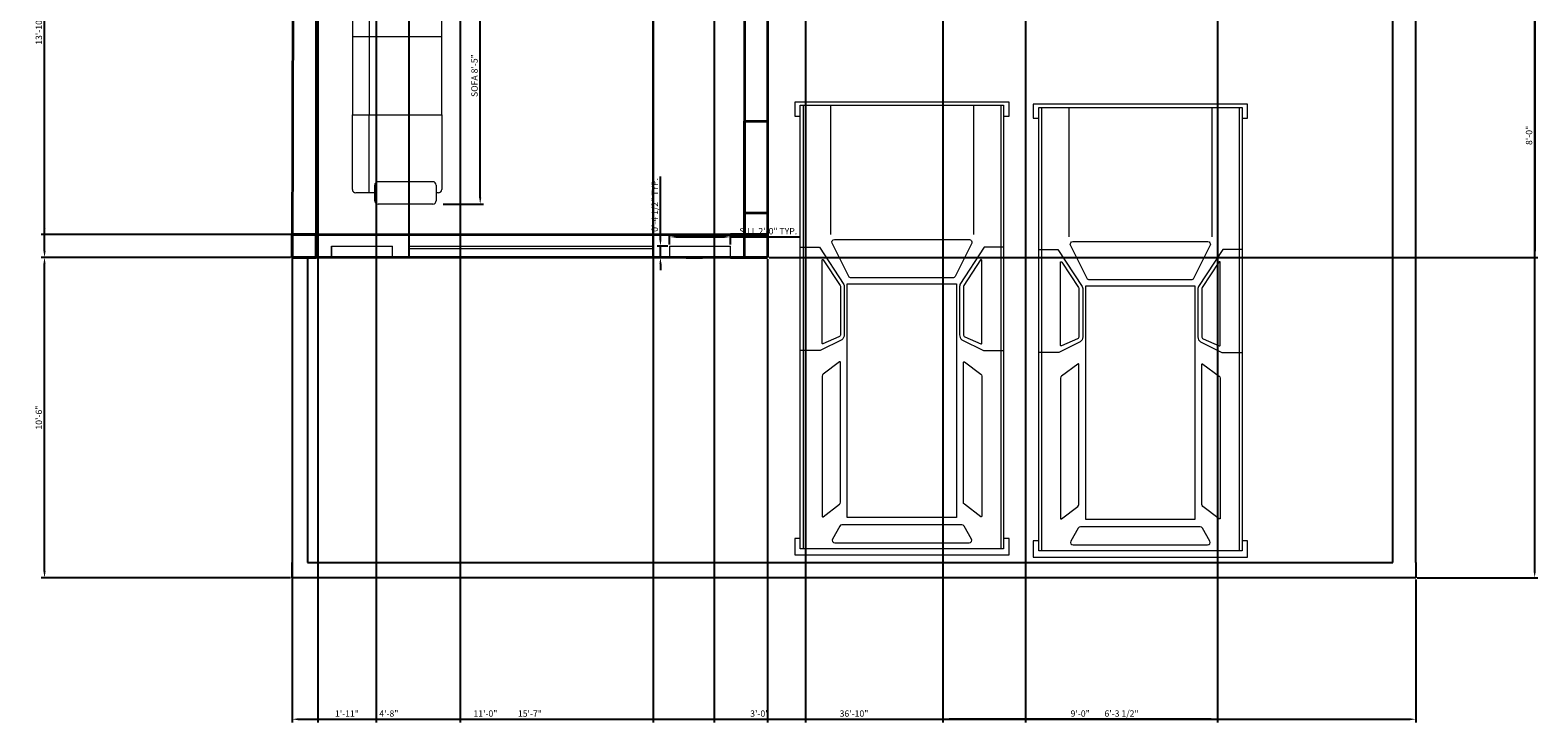
# Model space of a CAD drawing. Units: inches. Extents: x 1624 to 3956, y 1589 to 5028.
# Tile 1 of 16: x 1624 to 2218, y 1589 to 1862. Entities that reach past the tile are written whole.
import ezdxf

# ---------------------------------------------------------------- set-up
doc = ezdxf.new("R2010")
doc.units = ezdxf.units.IN
for name, color, linetype, lineweight in [('A-ANNO-DIMS', 2, 'Continuous', 13), ('A-COLS', 1, 'Continuous', 40), ('A-EQPM-VEHI', 8, 'Continuous', 13), ('A-FURN', 8, 'Continuous', 18), ('A-GLAZ', 4, 'Continuous', 18), ('A-WALL', 7, 'Continuous', 35), ('C-PROP', 7, 'Continuous', 25)]:
    doc.layers.add(name, color=color, linetype=linetype, lineweight=lineweight)
doc.styles.get("Standard").update_dxf_attribs({"font": 'arial.ttf'})
doc.dimstyles.new('Copy of ISO-25', dxfattribs={"dimtxt": 2.5, "dimasz": 2.5, "dimexe": 1.25, "dimexo": 0.625, "dimtad": 1, "dimdec": 1, "dimlunit": 4, "dimtxsty": 'Standard', "dimcen": 2.5, "dimadec": 0, "dimazin": 0, "dimtfac": 1, "dimtdec": 1, "dimtmove": 0, "dimatfit": 3, "dimfxl": 1, "dimarcsym": 0})

# ---------------------------------------------------------------- blocks, each defined once
blk = doc.blocks.new('*U16')
for p, q in [((32, 987), (4462, 987)), ((32, 715), (1324, 715)), ((32, -715), (1324, -715)), ((32, -987), (4462, -987))]:
    blk.add_line(p, q)
for points in [[(141, 1016), (141, 1071), (0, 1071), (0, -1071), (141, -1071), (141, -1016), (32, -1016), (32, 1016)], [(4362, 1016), (4462, 1016), (4462, -1016), (4362, -1016), (4362, -1071), (4525, -1071), (4525, 1071), (4362, 1071)], [(32, 1016), (4462, 1016), (4462, -1016), (32, -1016)], [(1815, 546), (4151, 546), (4151, -546), (1815, -546)]]:
    blk.add_lwpolyline(points, close=True)
for points in [[(1451, 1016), (1451, 823), (1822, 580, 0.086577), (1843, 576), (2326, 576, 0.227875), (2376, 600), (2482, 816), (2482, 1016)], [(1451, -1016), (1451, -823), (1822, -580, -0.086577), (1843, -576), (2326, -576, -0.227875), (2376, -600), (2482, -816), (2482, -1016)]]:
    blk.add_lwpolyline(points, format="xyb")
for points in [[(1577, 786), (1832, 618, 0.146139), (1846, 614), (2322, 614, 0.29766), (2345, 629), (2415, 789, 0.541236), (2409, 798), (1580, 798, 0.744989)], [(2596, 624), (2717, 787, -0.236929), (2737, 798), (4138, 798, -0.621576), (4143, 787), (4018, 624, -0.233368), (3998, 614), (2601, 614, -0.616908)], [(1410, 697), (1742, 531, -0.284287), (1756, 508), (1756, -508, -0.284287), (1742, -531), (1410, -697, -0.557284), (1373, -674), (1373, 674, -0.557284)], [(4366, 694), (4237, 622, 0.271143), (4224, 599), (4224, -599, 0.271143), (4237, -622), (4366, -694, 0.573387), (4404, -672), (4404, 672, 0.573387)], [(1577, -786), (1832, -618, -0.146139), (1846, -614), (2322, -614, -0.29766), (2345, -629), (2415, -789, -0.541236), (2409, -798), (1580, -798, -0.744989)], [(2596, -624), (2717, -787, 0.236929), (2737, -798), (4138, -798, 0.621576), (4143, -787), (4018, -624, 0.233368), (3998, -614), (2601, -614, 0.616908)]]:
    blk.add_lwpolyline(points, format="xyb", close=True)
blk = doc.blocks.new('A$C555E41E5')
for p, q in [((0.1, 0.6), (0.1, 0.77)), ((0.13, 0.8), (0.8, 0.8)), ((0.8, 0.8), (0.8, 0)), ((0.8, 0.8), (0.8, 0)), ((1.5, 0.8), (0.8, 0.8)), ((2.17, 0.8), (1.5, 0.8)), ((1.5, 0.8), (1.5, 0)), ((1.5, 0.8), (1.5, 0)), ((2.2, 0.6), (2.2, 0.77)), ((0, 0.08), (0, 0.57)), ((0.03, 0.6), (0.17, 0.6)), ((0.1, 0.65), (0.8, 0.65)), ((0.2, 0.08), (0.2, 0.57)), ((1.53, 0.65), (0.8, 0.65)), ((2.2, 0.65), (1.5, 0.65)), ((2.1, 0.08), (2.1, 0.57)), ((2.27, 0.6), (2.13, 0.6)), ((2.3, 0.08), (2.3, 0.57)), ((0.17, 0.05), (0.03, 0.05)), ((0.1, 0.03), (0.1, 0.05)), ((0.8, 0), (0.13, 0)), ((0.8, 0), (1.5, 0)), ((1.5, 0), (2.17, 0)), ((2.13, 0.05), (2.27, 0.05)), ((2.2, 0.03), (2.2, 0.05))]:
    blk.add_line(p, q)
for centre, start, end in [((0.13, 0.77), 90, 180), ((2.17, 0.77), 0, 90), ((0.03, 0.57), 90, 180), ((0.17, 0.57), 0, 90), ((2.13, 0.57), 90, 180), ((2.27, 0.57), 0, 90), ((0.03, 0.08), 180, 270), ((0.13, 0.03), 180, 270), ((0.17, 0.08), 270, 0), ((2.13, 0.08), 180, 270), ((2.17, 0.03), 270, 0), ((2.27, 0.08), 270, 0)]:
    blk.add_arc(centre, 0.03, start, end)
blk = doc.blocks.new('A$C2BCD7A6E')
blk.add_blockref('A$C555E41E5', (0, 0))
blk = doc.blocks.new('SILL-RECESS-24IN')
for p, q in [((0, 4.5), (0, 0)), ((0, 4.5), (24, 4.5)), ((24, 0), (24, 4.5))]:
    blk.add_line(p, q)
blk = doc.blocks.new('*D58')
at = {"layer": 'A-ANNO-DIMS', "color": 0, "lineweight": -2, "transparency": 16777216}
for p, q in [((1876.03, 1777.92), (1876.03, 1782.14)), ((1878.53, 1780.89), (1897.53, 1780.89)), ((1900.03, 1777.92), (1900.03, 1782.14)), ((1900.03, 1780.89), (1927.16, 1780.89))]:
    blk.add_line(p, q, dxfattribs=at)
at = {"layer": 'A-ANNO-DIMS', "color": 0, "transparency": 16777216}
for points in [[(1878.53, 1781.31), (1878.53, 1780.48), (1876.03, 1780.89)], [(1897.53, 1781.31), (1897.53, 1780.48), (1900.03, 1780.89)]]:
    blk.add_solid(points, dxfattribs=at)
at = {"layer": 'Defpoints', "color": 0, "transparency": 16777216}
for p in [(1900.03, 1780.89), (1876.03, 1777.29), (1900.03, 1777.29)]:
    blk.add_point(p, dxfattribs=at)
at = {"layer": 'A-ANNO-DIMS', "color": 0, "transparency": 16777216, "insert": (1914.84, 1782.81), "char_height": 2.5, "attachment_point": 5}
blk.add_mtext('SILL 2\'-0" TYP.', dxfattribs=at)
blk = doc.blocks.new('*D59')
at = {"layer": 'A-ANNO-DIMS', "color": 0, "lineweight": -2, "transparency": 16777216}
for p, q in [((1872.43, 1779.79), (1872.43, 1804.61)), ((1875.4, 1777.29), (1871.18, 1777.29)), ((1872.43, 1772.79), (1872.43, 1777.29)), ((1875.4, 1772.79), (1871.18, 1772.79)), ((1872.43, 1770.29), (1872.43, 1767.79))]:
    blk.add_line(p, q, dxfattribs=at)
at = {"layer": 'A-ANNO-DIMS', "color": 0, "transparency": 16777216}
for points in [[(1872.01, 1779.79), (1872.84, 1779.79), (1872.43, 1777.29)], [(1872.01, 1770.29), (1872.84, 1770.29), (1872.43, 1772.79)]]:
    blk.add_solid(points, dxfattribs=at)
at = {"layer": 'Defpoints', "color": 0, "transparency": 16777216}
for p in [(1872.43, 1777.29), (1876.03, 1777.29), (1876.03, 1772.79)]:
    blk.add_point(p, dxfattribs=at)
at = {"layer": 'A-ANNO-DIMS', "color": 0, "transparency": 16777216, "insert": (1870.51, 1793.45), "char_height": 2.5, "attachment_point": 5, "rotation": 90}
blk.add_mtext('0\'-4 1/2" TYP.', dxfattribs=at)
blk = doc.blocks.new('*D64')
at = {"layer": 'A-ANNO-DIMS', "color": 0, "lineweight": -2, "transparency": 16777216}
for p, q in [((1787, 1894.81), (1802.77, 1894.81)), ((1801.52, 1796.3), (1801.52, 1892.31)), ((1787, 1793.8), (1802.77, 1793.8))]:
    blk.add_line(p, q, dxfattribs=at)
at = {"layer": 'A-ANNO-DIMS', "color": 0, "transparency": 16777216}
for points in [[(1801.11, 1892.31), (1801.94, 1892.31), (1801.52, 1894.81)], [(1801.11, 1796.3), (1801.94, 1796.3), (1801.52, 1793.8)]]:
    blk.add_solid(points, dxfattribs=at)
at = {"layer": 'Defpoints', "color": 0, "transparency": 16777216}
for p in [(1786.37, 1894.81), (1801.52, 1894.81), (1786.37, 1793.8)]:
    blk.add_point(p, dxfattribs=at)
at = {"layer": 'A-ANNO-DIMS', "color": 0, "transparency": 16777216, "insert": (1799.6, 1844.31), "char_height": 2.5, "attachment_point": 5, "rotation": 90}
blk.add_mtext('SOFA 8\'-5"', dxfattribs=at)
blk = doc.blocks.new('*D66')
at = {"layer": 'A-ANNO-DIMS', "color": 0, "lineweight": -2, "transparency": 16777216}
for p, q in [((1727.58, 1646.17), (1727.58, 1589.9)), ((2169.58, 1646.17), (2169.58, 1589.9)), ((1730.08, 1591.15), (2167.08, 1591.15))]:
    blk.add_line(p, q, dxfattribs=at)
at = {"layer": 'A-ANNO-DIMS', "color": 0, "transparency": 16777216}
for points in [[(1730.08, 1591.57), (1730.08, 1590.73), (1727.58, 1591.15)], [(2167.08, 1591.57), (2167.08, 1590.73), (2169.58, 1591.15)]]:
    blk.add_solid(points, dxfattribs=at)
at = {"layer": 'Defpoints', "color": 0, "transparency": 16777216}
for p in [(1727.58, 1646.79), (2169.58, 1646.79), (2169.58, 1591.15)]:
    blk.add_point(p, dxfattribs=at)
at = {"layer": 'A-ANNO-DIMS', "color": 0, "transparency": 16777216, "insert": (1948.58, 1593.05), "char_height": 2.5, "attachment_point": 5}
blk.add_mtext('36\'-10"', dxfattribs=at)
blk = doc.blocks.new('*D67')
at = {"layer": 'A-ANNO-DIMS', "color": 0, "lineweight": -2, "transparency": 16777216}
for p, q in [((2170.2, 2564.79), (2217.63, 2564.79)), ((2216.38, 1649.29), (2216.38, 2562.29)), ((2170.2, 1646.79), (2217.63, 1646.79))]:
    blk.add_line(p, q, dxfattribs=at)
at = {"layer": 'A-ANNO-DIMS', "color": 0, "transparency": 16777216}
for points in [[(2215.96, 2562.29), (2216.8, 2562.29), (2216.38, 2564.79)], [(2215.96, 1649.29), (2216.8, 1649.29), (2216.38, 1646.79)]]:
    blk.add_solid(points, dxfattribs=at)
at = {"layer": 'Defpoints', "color": 0, "transparency": 16777216}
for p in [(2169.58, 2564.79), (2216.38, 2564.79), (2169.58, 1646.79)]:
    blk.add_point(p, dxfattribs=at)
at = {"layer": 'A-ANNO-DIMS', "color": 0, "transparency": 16777216, "insert": (2214.48, 2105.79), "char_height": 2.5, "attachment_point": 5, "rotation": 90}
blk.add_mtext('76\'-6"', dxfattribs=at)
blk = doc.blocks.new('*D69')
at = {"layer": 'A-ANNO-DIMS', "color": 0, "lineweight": -2, "transparency": 16777216}
for p, q in [((1727.95, 2495.79), (1628.86, 2495.79)), ((1630.11, 1775.29), (1630.11, 2493.29)), ((1726.95, 1772.79), (1628.86, 1772.79))]:
    blk.add_line(p, q, dxfattribs=at)
at = {"layer": 'A-ANNO-DIMS', "color": 0, "transparency": 16777216}
for points in [[(1629.69, 2493.29), (1630.53, 2493.29), (1630.11, 2495.79)], [(1629.69, 1775.29), (1630.53, 1775.29), (1630.11, 1772.79)]]:
    blk.add_solid(points, dxfattribs=at)
at = {"layer": 'Defpoints', "color": 0, "transparency": 16777216}
for p in [(1630.11, 2495.79), (1728.58, 2495.79), (1727.58, 1772.79)]:
    blk.add_point(p, dxfattribs=at)
at = {"layer": 'A-ANNO-DIMS', "color": 0, "transparency": 16777216, "insert": (1628.21, 2134.29), "char_height": 2.5, "attachment_point": 5, "rotation": 90}
blk.add_mtext('60\'-3"', dxfattribs=at)
blk = doc.blocks.new('*D70')
at = {"layer": 'A-ANNO-DIMS', "color": 0, "lineweight": -2, "transparency": 16777216}
for p, q in [((1726.95, 1772.79), (1628.86, 1772.79)), ((1630.11, 1649.29), (1630.11, 1770.29)), ((1726.95, 1646.79), (1628.86, 1646.79))]:
    blk.add_line(p, q, dxfattribs=at)
at = {"layer": 'A-ANNO-DIMS', "color": 0, "transparency": 16777216}
for points in [[(1629.69, 1770.29), (1630.53, 1770.29), (1630.11, 1772.79)], [(1629.69, 1649.29), (1630.53, 1649.29), (1630.11, 1646.79)]]:
    blk.add_solid(points, dxfattribs=at)
at = {"layer": 'Defpoints', "color": 0, "transparency": 16777216}
for p in [(1630.11, 1772.79), (1727.58, 1772.79), (1727.58, 1646.79)]:
    blk.add_point(p, dxfattribs=at)
at = {"layer": 'A-ANNO-DIMS', "color": 0, "transparency": 16777216, "insert": (1628.21, 1709.79), "char_height": 2.5, "attachment_point": 5, "rotation": 90}
blk.add_mtext('10\'-6"', dxfattribs=at)
blk = doc.blocks.new('*D73')
at = {"layer": 'A-ANNO-DIMS', "color": 0, "lineweight": -2, "transparency": 16777216}
for p, q in [((1727.58, 1772.17), (1727.58, 1589.9)), ((1914.58, 1772.17), (1914.58, 1589.9)), ((1730.08, 1591.15), (1912.08, 1591.15))]:
    blk.add_line(p, q, dxfattribs=at)
at = {"layer": 'A-ANNO-DIMS', "color": 0, "transparency": 16777216}
for points in [[(1730.08, 1591.57), (1730.08, 1590.73), (1727.58, 1591.15)], [(1912.08, 1591.57), (1912.08, 1590.73), (1914.58, 1591.15)]]:
    blk.add_solid(points, dxfattribs=at)
at = {"layer": 'Defpoints', "color": 0, "transparency": 16777216}
for p in [(1727.58, 1772.79), (1914.58, 1772.79), (1914.58, 1591.15)]:
    blk.add_point(p, dxfattribs=at)
at = {"layer": 'A-ANNO-DIMS', "color": 0, "transparency": 16777216, "insert": (1821.08, 1593.05), "char_height": 2.5, "attachment_point": 5}
blk.add_mtext('15\'-7"', dxfattribs=at)
blk = doc.blocks.new('*D74')
at = {"layer": 'A-ANNO-DIMS', "color": 0, "lineweight": -2, "transparency": 16777216}
for p, q in [((1915.2, 1868.79), (2217.63, 1868.79)), ((2216.38, 1866.29), (2216.38, 1775.29)), ((1915.2, 1772.79), (2217.63, 1772.79))]:
    blk.add_line(p, q, dxfattribs=at)
at = {"layer": 'A-ANNO-DIMS', "color": 0, "transparency": 16777216}
for points in [[(2215.96, 1866.29), (2216.8, 1866.29), (2216.38, 1868.79)], [(2215.96, 1775.29), (2216.8, 1775.29), (2216.38, 1772.79)]]:
    blk.add_solid(points, dxfattribs=at)
at = {"layer": 'Defpoints', "color": 0, "transparency": 16777216}
for p in [(1914.58, 1868.79), (1914.58, 1772.79), (2216.38, 1772.79)]:
    blk.add_point(p, dxfattribs=at)
at = {"layer": 'A-ANNO-DIMS', "color": 0, "transparency": 16777216, "insert": (2214.48, 1820.79), "char_height": 2.5, "attachment_point": 5, "rotation": 90}
blk.add_mtext('8\'-0"', dxfattribs=at)
blk = doc.blocks.new('*D75')
at = {"layer": 'A-ANNO-DIMS', "color": 0, "lineweight": -2, "transparency": 16777216}
for p, q in [((1737.58, 2486.17), (1737.58, 1589.9)), ((1793.58, 2486.17), (1793.58, 1589.9)), ((1740.08, 1591.15), (1791.08, 1591.15))]:
    blk.add_line(p, q, dxfattribs=at)
at = {"layer": 'A-ANNO-DIMS', "color": 0, "transparency": 16777216}
for points in [[(1740.08, 1591.57), (1740.08, 1590.73), (1737.58, 1591.15)], [(1791.08, 1591.57), (1791.08, 1590.73), (1793.58, 1591.15)]]:
    blk.add_solid(points, dxfattribs=at)
at = {"layer": 'Defpoints', "color": 0, "transparency": 16777216}
for p in [(1737.58, 2486.79), (1793.58, 2486.79), (1793.58, 1591.15)]:
    blk.add_point(p, dxfattribs=at)
at = {"layer": 'A-ANNO-DIMS', "color": 0, "transparency": 16777216, "insert": (1765.58, 1593.05), "char_height": 2.5, "attachment_point": 5}
blk.add_mtext('4\'-8"', dxfattribs=at)
blk = doc.blocks.new('*D82')
at = {"layer": 'A-ANNO-DIMS', "color": 0, "lineweight": -2, "transparency": 16777216}
for p, q in [((1737.58, 2306.17), (1737.58, 1589.9)), ((1869.56, 2306.17), (1869.56, 1589.9)), ((1740.08, 1591.15), (1867.06, 1591.15))]:
    blk.add_line(p, q, dxfattribs=at)
at = {"layer": 'A-ANNO-DIMS', "color": 0, "transparency": 16777216}
for points in [[(1740.08, 1591.57), (1740.08, 1590.73), (1737.58, 1591.15)], [(1867.06, 1591.57), (1867.06, 1590.73), (1869.56, 1591.15)]]:
    blk.add_solid(points, dxfattribs=at)
at = {"layer": 'Defpoints', "color": 0, "transparency": 16777216}
for p in [(1737.58, 2306.79), (1869.56, 2306.79), (1869.56, 1591.15)]:
    blk.add_point(p, dxfattribs=at)
at = {"layer": 'A-ANNO-DIMS', "color": 0, "transparency": 16777216, "insert": (1803.57, 1593.05), "char_height": 2.5, "attachment_point": 5}
blk.add_mtext('11\'-0"', dxfattribs=at)
blk = doc.blocks.new('*D84')
at = {"layer": 'A-ANNO-DIMS', "color": 0, "lineweight": -2, "transparency": 16777216}
for p, q in [((1904.9, 1948.29), (1628.86, 1948.29)), ((1630.11, 1784.29), (1630.11, 1945.79)), ((1904.9, 1781.79), (1628.86, 1781.79))]:
    blk.add_line(p, q, dxfattribs=at)
at = {"layer": 'A-ANNO-DIMS', "color": 0, "transparency": 16777216}
for points in [[(1629.69, 1945.79), (1630.53, 1945.79), (1630.11, 1948.29)], [(1629.69, 1784.29), (1630.53, 1784.29), (1630.11, 1781.79)]]:
    blk.add_solid(points, dxfattribs=at)
at = {"layer": 'Defpoints', "color": 0, "transparency": 16777216}
for p in [(1630.11, 1948.29), (1905.53, 1948.29), (1905.53, 1781.79)]:
    blk.add_point(p, dxfattribs=at)
at = {"layer": 'A-ANNO-DIMS', "color": 0, "transparency": 16777216, "insert": (1628.19, 1865.04), "char_height": 2.5, "attachment_point": 5, "rotation": 90}
blk.add_mtext('13\'-10 1/2"', dxfattribs=at)
blk = doc.blocks.new('*D85')
at = {"layer": 'A-ANNO-DIMS', "color": 0, "lineweight": -2, "transparency": 16777216}
for p, q in [((1983.58, 1877.17), (1983.58, 1589.9)), ((2091.58, 1877.17), (2091.58, 1589.9)), ((2089.08, 1591.15), (1986.08, 1591.15))]:
    blk.add_line(p, q, dxfattribs=at)
at = {"layer": 'A-ANNO-DIMS', "color": 0, "transparency": 16777216}
for points in [[(1986.08, 1591.57), (1986.08, 1590.73), (1983.58, 1591.15)], [(2089.08, 1591.57), (2089.08, 1590.73), (2091.58, 1591.15)]]:
    blk.add_solid(points, dxfattribs=at)
at = {"layer": 'Defpoints', "color": 0, "transparency": 16777216}
for p in [(1983.58, 1877.79), (2091.58, 1877.79), (1983.58, 1591.15)]:
    blk.add_point(p, dxfattribs=at)
at = {"layer": 'A-ANNO-DIMS', "color": 0, "transparency": 16777216, "insert": (2037.58, 1593.05), "char_height": 2.5, "attachment_point": 5}
blk.add_mtext('9\'-0"', dxfattribs=at)
blk = doc.blocks.new('*D92')
at = {"layer": 'A-ANNO-DIMS', "color": 0, "lineweight": -2, "transparency": 16777216}
for p, q in [((2016.08, 2072.17), (2016.08, 1589.9)), ((2091.58, 2072.17), (2091.58, 1589.9)), ((2018.58, 1591.15), (2089.08, 1591.15))]:
    blk.add_line(p, q, dxfattribs=at)
at = {"layer": 'A-ANNO-DIMS', "color": 0, "transparency": 16777216}
for points in [[(2018.58, 1591.57), (2018.58, 1590.73), (2016.08, 1591.15)], [(2089.08, 1591.57), (2089.08, 1590.73), (2091.58, 1591.15)]]:
    blk.add_solid(points, dxfattribs=at)
at = {"layer": 'Defpoints', "color": 0, "transparency": 16777216}
for p in [(2016.08, 2072.79), (2091.58, 2072.79), (2091.58, 1591.15)]:
    blk.add_point(p, dxfattribs=at)
at = {"layer": 'A-ANNO-DIMS', "color": 0, "transparency": 16777216, "insert": (2053.83, 1593.07), "char_height": 2.5, "attachment_point": 5}
blk.add_mtext('6\'-3 1/2"', dxfattribs=at)
blk = doc.blocks.new('*D94')
at = {"layer": 'A-ANNO-DIMS', "color": 0, "lineweight": -2, "transparency": 16777216}
for p, q in [((1893.52, 2315.17), (1893.52, 1589.9)), ((1929.52, 2315.17), (1929.52, 1589.9)), ((1896.02, 1591.15), (1927.02, 1591.15))]:
    blk.add_line(p, q, dxfattribs=at)
at = {"layer": 'A-ANNO-DIMS', "color": 0, "transparency": 16777216}
for points in [[(1896.02, 1591.57), (1896.02, 1590.73), (1893.52, 1591.15)], [(1927.02, 1591.57), (1927.02, 1590.73), (1929.52, 1591.15)]]:
    blk.add_solid(points, dxfattribs=at)
at = {"layer": 'Defpoints', "color": 0, "transparency": 16777216}
for p in [(1893.52, 2315.79), (1929.52, 2315.79), (1929.52, 1591.15)]:
    blk.add_point(p, dxfattribs=at)
at = {"layer": 'A-ANNO-DIMS', "color": 0, "transparency": 16777216, "insert": (1911.52, 1593.05), "char_height": 2.5, "attachment_point": 5}
blk.add_mtext('3\'-0"', dxfattribs=at)
blk = doc.blocks.new('*D97')
at = {"layer": 'A-ANNO-DIMS', "color": 0, "lineweight": -2, "transparency": 16777216}
for p, q in [((1773.53, 1773.42), (1773.53, 2612.84)), ((1776.03, 2611.59), (1867.03, 2611.59)), ((1869.53, 1773.42), (1869.53, 2612.84))]:
    blk.add_line(p, q, dxfattribs=at)
at = {"layer": 'A-ANNO-DIMS', "color": 0, "transparency": 16777216}
for points in [[(1776.03, 2612.01), (1776.03, 2611.18), (1773.53, 2611.59)], [(1867.03, 2612.01), (1867.03, 2611.18), (1869.53, 2611.59)]]:
    blk.add_solid(points, dxfattribs=at)
at = {"layer": 'Defpoints', "color": 0, "transparency": 16777216}
for p in [(1869.53, 2611.59), (1773.53, 1772.79), (1869.53, 1772.79)]:
    blk.add_point(p, dxfattribs=at)
at = {"layer": 'A-ANNO-DIMS', "color": 0, "transparency": 16777216, "insert": (1821.53, 2613.5), "char_height": 2.5, "attachment_point": 5}
blk.add_mtext('8\'-0"', dxfattribs=at)
blk = doc.blocks.new('*D99')
at = {"layer": 'A-ANNO-DIMS', "color": 0, "lineweight": -2, "transparency": 16777216}
for p, q in [((1737.58, 2239.75), (1737.58, 1589.9)), ((1760.58, 2239.75), (1760.58, 1589.9)), ((1740.08, 1591.15), (1758.08, 1591.15))]:
    blk.add_line(p, q, dxfattribs=at)
at = {"layer": 'A-ANNO-DIMS', "color": 0, "transparency": 16777216}
for points in [[(1740.08, 1591.57), (1740.08, 1590.73), (1737.58, 1591.15)], [(1758.08, 1591.57), (1758.08, 1590.73), (1760.58, 1591.15)]]:
    blk.add_solid(points, dxfattribs=at)
at = {"layer": 'Defpoints', "color": 0, "transparency": 16777216}
for p in [(1737.58, 2240.37), (1760.58, 2240.37), (1760.58, 1591.15)]:
    blk.add_point(p, dxfattribs=at)
at = {"layer": 'A-ANNO-DIMS', "color": 0, "transparency": 16777216, "insert": (1749.08, 1593.03), "char_height": 2.5, "attachment_point": 5}
blk.add_mtext('1\'-11"', dxfattribs=at)
blk = doc.blocks.new('*D101')
at = {"layer": 'A-ANNO-DIMS', "color": 0, "lineweight": -2, "transparency": 16777216}
for p, q in [((1737.01, 1782.42), (1737.01, 2612.84)), ((1739.51, 2611.59), (1771.03, 2611.59)), ((1773.53, 1782.42), (1773.53, 2612.84))]:
    blk.add_line(p, q, dxfattribs=at)
at = {"layer": 'A-ANNO-DIMS', "color": 0, "transparency": 16777216}
for points in [[(1739.51, 2612.01), (1739.51, 2611.18), (1737.01, 2611.59)], [(1771.03, 2612.01), (1771.03, 2611.18), (1773.53, 2611.59)]]:
    blk.add_solid(points, dxfattribs=at)
at = {"layer": 'Defpoints', "color": 0, "transparency": 16777216}
for p in [(1773.53, 2611.59), (1737.01, 1781.79), (1773.53, 1781.79)]:
    blk.add_point(p, dxfattribs=at)
at = {"layer": 'A-ANNO-DIMS', "color": 0, "transparency": 16777216, "insert": (1755.27, 2613.51), "char_height": 2.5, "attachment_point": 5}
blk.add_mtext('3\'-0 1/2"', dxfattribs=at)

msp = doc.modelspace()

# ---------------------------------------------------------------- linework, layer by layer
at = {"layer": 'A-COLS'}
for p, q in [((1727.6, 1781.79), (1727.58, 1772.79)), ((1737.01, 1781.79), (1727.6, 1781.79)), ((1737.01, 1781.79), (1737.01, 1772.79)), ((1737.01, 1772.79), (1737.01, 1781.79)), ((1905.53, 1781.79), (1914.58, 1781.79)), ((1727.58, 1772.79), (1737.01, 1772.79))]:
    msp.add_line(p, q, dxfattribs=at)
at = {"layer": 'A-GLAZ'}
for p, q in [((1767.03, 1781.79), (1743.03, 1781.79)), ((1869.53, 1781.79), (1773.53, 1781.79)), ((1773.53, 1781.79), (1773.53, 1772.79)), ((1869.53, 1772.79), (1869.53, 1781.79)), ((1900.03, 1781.79), (1876.03, 1781.79)), ((1743.03, 1772.79), (1743.03, 1777.29)), ((1773.53, 1777.29), (1869.53, 1777.29)), ((1773.53, 1776.29), (1869.53, 1776.29))]:
    msp.add_line(p, q, dxfattribs=at)
at = {"layer": 'A-WALL'}
for p, q in [((1728.58, 2301.8), (1727.58, 1772.79)), ((1737.01, 1948.29), (1737.01, 1781.79)), ((1905.53, 1948.29), (1905.53, 1781.79)), ((1914.58, 1868.79), (1914.58, 1772.79)), ((1905.53, 1790.34), (1905.53, 1826.34)), ((1905.53, 1826.34), (1914.58, 1826.34)), ((1905.53, 1781.79), (1905.53, 1790.34)), ((1905.53, 1790.34), (1914.58, 1790.34)), ((1727.58, 1772.79), (1727.58, 1781.79)), ((1727.58, 1781.79), (1727.6, 1781.79)), ((1737.01, 1781.79), (1905.53, 1781.79)), ((1905.53, 1781.79), (1900.03, 1781.79)), ((1905.53, 1772.79), (1905.53, 1781.79)), ((1914.58, 1772.79), (1727.58, 1772.79)), ((1743.03, 1772.79), (1736.53, 1772.79)), ((1773.53, 1772.79), (1767.03, 1772.79)), ((1881.53, 1772.79), (1785.53, 1772.79)), ((1876.03, 1772.79), (1869.53, 1772.79)), ((1882.53, 1772.79), (1889.03, 1772.79)), ((1900.03, 1772.79), (1905.53, 1772.79)), ((1905.53, 1772.79), (1914.58, 1772.79))]:
    msp.add_line(p, q, dxfattribs=at)
at = {"layer": 'C-PROP'}
for p, q in [((2169.58, 1652.79), (2169.58, 2559.46)), ((2160.58, 1652.79), (2160.58, 2555.79)), ((1727.58, 1772.79), (1727.58, 1652.79)), ((1733.58, 1772.79), (1733.58, 1652.79)), ((1727.58, 1646.79), (1727.58, 1652.79)), ((1733.58, 1652.79), (2100.58, 1652.79)), ((2100.58, 1652.79), (2160.58, 1652.79)), ((2169.58, 1652.79), (2169.58, 1646.79)), ((2169.58, 1646.79), (1727.58, 1646.79))]:
    msp.add_line(p, q, dxfattribs=at)

# ---------------------------------------------------------------- block references
at = {"layer": 'A-EQPM-VEHI', "xscale": 0.0393700787401575, "yscale": 0.0393700787401575, "zscale": 0.0393700787401575, "rotation": 270}
for p in [(1967.44, 1833.91), (2061.24, 1833.08), (2061.24, 1833.08)]:
    msp.add_blockref('*U16', p, dxfattribs=at)
at = {"layer": 'A-FURN', "xscale": 43.92080760397013, "yscale": 43.92080760397013, "zscale": 43.92080760397013, "rotation": 90}
msp.add_blockref('A$C2BCD7A6E', (1786.37, 1793.8), dxfattribs=at)
at = {"layer": 'A-GLAZ'}
for p in [(1743.03, 1772.79), (1876.03, 1772.79)]:
    msp.add_blockref('SILL-RECESS-24IN', p, dxfattribs=at)

# ---------------------------------------------------------------- dimensions: what is measured, and where the dimension line sits
at = {"layer": 'A-ANNO-DIMS'}
for base, p1, p2, picture, middle in [((1773.53, 2611.59), (1737.01, 1781.79), (1773.53, 1781.79), '*D101', (1755.27, 2613.51)), ((1869.53, 2611.59), (1773.53, 1772.79), (1869.53, 1772.79), '*D97', (1821.53, 2613.5)), ((1793.58, 1591.15), (1737.58, 2486.79), (1793.58, 2486.79), '*D75', (1765.58, 1593.05)), ((1929.52, 1591.15), (1893.52, 2315.79), (1929.52, 2315.79), '*D94', (1911.52, 1593.05)), ((1869.56, 1591.15), (1737.58, 2306.79), (1869.56, 2306.79), '*D82', (1803.57, 1593.05)), ((1760.58, 1591.15), (1737.58, 2240.37), (1760.58, 2240.37), '*D99', (1749.08, 1593.03)), ((2091.58, 1591.15), (2016.08, 2072.79), (2091.58, 2072.79), '*D92', (2053.83, 1593.07)), ((1983.58, 1591.15), (2091.58, 1877.79), (1983.58, 1877.79), '*D85', (2037.58, 1593.05)), ((1914.58, 1591.15), (1727.58, 1772.79), (1914.58, 1772.79), '*D73', (1821.08, 1593.05)), ((2169.58, 1591.15), (1727.58, 1646.79), (2169.58, 1646.79), '*D66', (1948.58, 1593.05))]:
    dim = msp.add_linear_dim(base=base, p1=p1, p2=p2, dimstyle='Copy of ISO-25', override={"dimdec": 1, "dimlfac": 1, "dimrnd": 0, "dimzin": 1, "dimdsep": 46, "dimlunit": 4, "dimfrac": 2}, dxfattribs=at)
    dim.commit()
    dim.dimension.update_dxf_attribs({"geometry": picture, "text_midpoint": middle})
for base, p1, p2, picture, middle in [((2216.38, 2564.79), (2169.58, 1646.79), (2169.58, 2564.79), '*D67', (2214.48, 2105.79)), ((1630.11, 2495.79), (1727.58, 1772.79), (1728.58, 2495.79), '*D69', (1628.21, 2134.29)), ((1630.11, 1948.29), (1905.53, 1781.79), (1905.53, 1948.29), '*D84', (1628.19, 1865.04)), ((2216.38, 1772.79), (1914.58, 1868.79), (1914.58, 1772.79), '*D74', (2214.48, 1820.79)), ((1630.11, 1772.79), (1727.58, 1646.79), (1727.58, 1772.79), '*D70', (1628.21, 1709.79))]:
    dim = msp.add_linear_dim(base=base, p1=p1, p2=p2, angle=90, dimstyle='Copy of ISO-25', override={"dimdec": 1, "dimlfac": 1, "dimrnd": 0, "dimzin": 1, "dimdsep": 46, "dimlunit": 4, "dimfrac": 2}, dxfattribs=at)
    dim.commit()
    dim.dimension.update_dxf_attribs({"geometry": picture, "text_midpoint": middle})
for base, p1, p2, text, picture, middle in [((1801.52, 1894.81), (1786.37, 1793.8), (1786.37, 1894.81), 'SOFA <>', '*D64', (1799.6, 1844.31)), ((1872.43, 1777.29), (1876.03, 1772.79), (1876.03, 1777.29), '<> TYP.', '*D59', (1870.51, 1793.45))]:
    dim = msp.add_linear_dim(base=base, p1=p1, p2=p2, angle=90, text=text, dimstyle='Copy of ISO-25', override={"dimdec": 1, "dimlfac": 1, "dimrnd": 0, "dimzin": 1, "dimdsep": 46, "dimlunit": 4, "dimfrac": 2}, dxfattribs=at)
    dim.commit()
    dim.dimension.update_dxf_attribs({"geometry": picture, "text_midpoint": middle})
dim = msp.add_linear_dim(base=(1900.03, 1780.89), p1=(1876.03, 1777.29), p2=(1900.03, 1777.29), text='SILL <> TYP.', dimstyle='Copy of ISO-25', override={"dimdec": 1, "dimlfac": 1, "dimrnd": 0, "dimzin": 1, "dimdsep": 46, "dimlunit": 4, "dimfrac": 2}, dxfattribs=at)
dim.commit()
dim.dimension.update_dxf_attribs({"geometry": '*D58', "text_midpoint": (1914.84, 1782.81)})

doc.saveas('drawing.dxf')
